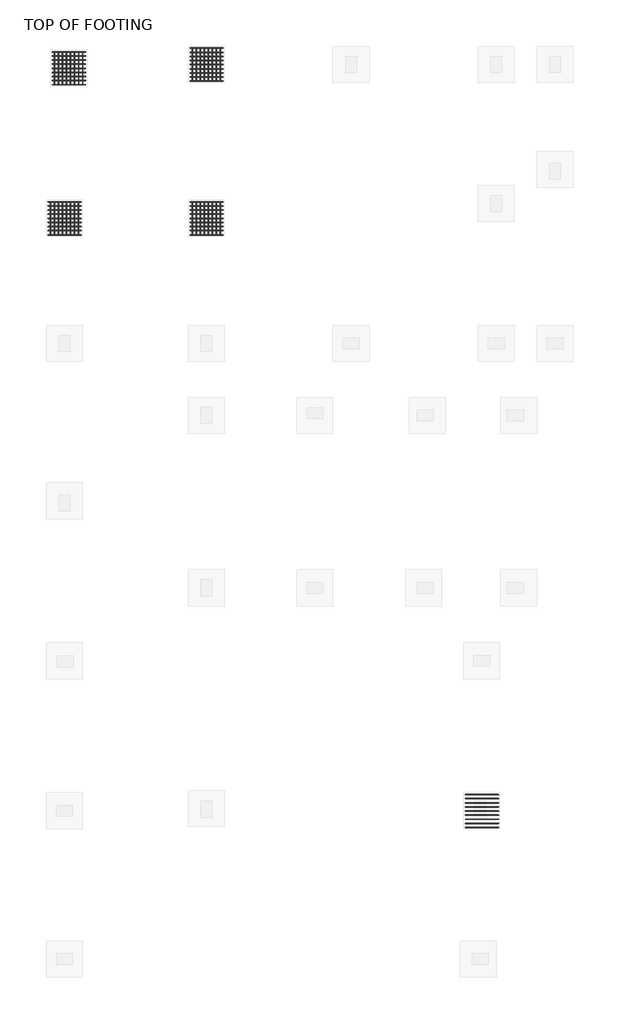
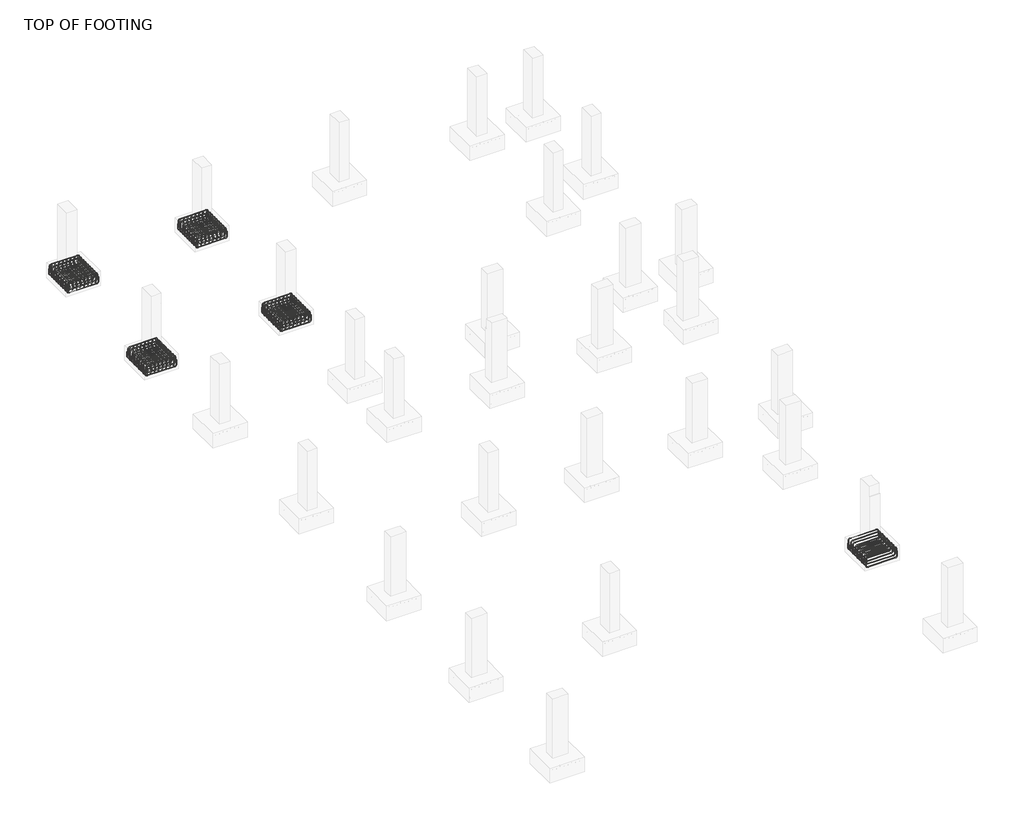
# One storey, part 13 of 20: 18 reinforcing bars.
"""IFC4 building model written with IfcOpenShell, lengths in millimetres."""

from ifc_helpers import new_model, si_unit, point, frame, origin, place, context, project, spatial, polyline, circle_curve, trimmed, segment, composite_curve, source, transform, mapped, element, save
from ifc_brep_helpers import swept_disk

model = new_model("IFC4")

# Units and contexts
model_context = context("Model", 3, world=origin())
ifc_project = project(units=[si_unit("LENGTHUNIT", "METRE", prefix="MILLI")], contexts=[model_context])

# Site, building, storey
site = spatial("IfcSite", under=ifc_project)
building = spatial("IfcBuilding", under=site)
storey = spatial("IfcBuildingStorey", under=building, Name="TOP OF FOOTING", Elevation=-1828.8)

# Reinforcing bars
placement = place(None, origin())
reinforcing_bar_shape = source(origin(), model_context, "Body", "SolidModel", [
    swept_disk(composite_curve([segment(polyline([(-5168.1365686, 22041.4849362, -2006.6587682), (-5168.1365686, 22041.4849362, -2153.9587682)]), True, "CONTINUOUS"), segment(trimmed(circle_curve(frame((-5214.4865686, 22041.4849362, -2153.9587682), z_axis=(0.0, 1.0, 0.0), x_axis=(46.350000000000364, 0.0, 0.0)), 46.35), [point((-5168.1365686, 22041.4849362, -2153.9587682))], [point((-5214.4865686, 22041.4849362, -2200.3087682))], True, "CARTESIAN"), True, "CONTINUOUS"), segment(polyline([(-5214.4865686, 22041.4849362, -2200.3087682), (-6029.0865686, 22041.4849362, -2200.3087682)]), True, "CONTINUOUS"), segment(trimmed(circle_curve(frame((-6029.0865686, 22041.4849362, -2153.9587682), z_axis=(0.0, 1.0, 0.0), x_axis=(0.0, 0.0, -46.34999999999991)), 46.35), [point((-6029.0865686, 22041.4849362, -2200.3087682))], [point((-6075.4365686, 22041.4849362, -2153.9587682))], True, "CARTESIAN"), True, "CONTINUOUS"), segment(polyline([(-6075.4365686, 22041.4849362, -2153.9587682), (-6075.4365686, 22041.4849362, -2006.6587682)]), True, "CONTINUOUS")], self_intersect=False), 6.35),
])
element("IfcReinforcingBar", 1, at=placement, inside=storey, context=model_context, shape_type="MappedRepresentation", body=[
    mapped(reinforcing_bar_shape, transform((0.0, 0.0, 0.0), x_axis=(1.0, 0.0, 0.0), y_axis=(0.0, 1.0, 0.0), z_axis=(0.0, 0.0, 1.0))),
    mapped(reinforcing_bar_shape, transform((0.0, -113.4125, 0.0), x_axis=(1.0, 0.0, 0.0), y_axis=(0.0, 1.0, 0.0), z_axis=(0.0, 0.0, 1.0))),
    mapped(reinforcing_bar_shape, transform((0.0, -226.825, 0.0), x_axis=(1.0, 0.0, 0.0), y_axis=(0.0, 1.0, 0.0), z_axis=(0.0, 0.0, 1.0))),
    mapped(reinforcing_bar_shape, transform((0.0, -340.2375, 0.0), x_axis=(1.0, 0.0, 0.0), y_axis=(0.0, 1.0, 0.0), z_axis=(0.0, 0.0, 1.0))),
    mapped(reinforcing_bar_shape, transform((0.0, -453.65, 0.0), x_axis=(1.0, 0.0, 0.0), y_axis=(0.0, 1.0, 0.0), z_axis=(0.0, 0.0, 1.0))),
    mapped(reinforcing_bar_shape, transform((0.0, -567.0625, 0.0), x_axis=(1.0, 0.0, 0.0), y_axis=(0.0, 1.0, 0.0), z_axis=(0.0, 0.0, 1.0))),
    mapped(reinforcing_bar_shape, transform((0.0, -680.475, 0.0), x_axis=(1.0, 0.0, 0.0), y_axis=(0.0, 1.0, 0.0), z_axis=(0.0, 0.0, 1.0))),
    mapped(reinforcing_bar_shape, transform((0.0, -793.8875, 0.0), x_axis=(1.0, 0.0, 0.0), y_axis=(0.0, 1.0, 0.0), z_axis=(0.0, 0.0, 1.0))),
    mapped(reinforcing_bar_shape, transform((0.0, -907.3, 0.0), x_axis=(1.0, 0.0, 0.0), y_axis=(0.0, 1.0, 0.0), z_axis=(0.0, 0.0, 1.0))),
])
reinforcing_bar_2_shape = source(origin(), model_context, "Body", "SolidModel", [
    swept_disk(composite_curve([segment(polyline([(-6055.9624573, 22041.4849362, -2068.8), (-6055.9624573, 22041.4849362, -1921.5)]), True, "CONTINUOUS"), segment(trimmed(circle_curve(frame((-6009.6124573, 22041.4849362, -1921.5), z_axis=(0.0, 1.0, 0.0), x_axis=(-46.350000000000364, 0.0, 0.0)), 46.35), [point((-6055.9624573, 22041.4849362, -1921.5))], [point((-6009.6124573, 22041.4849362, -1875.15))], True, "CARTESIAN"), True, "CONTINUOUS"), segment(polyline([(-6009.6124573, 22041.4849362, -1875.15), (-5240.1490576, 22041.4849362, -1875.15)]), True, "CONTINUOUS"), segment(trimmed(circle_curve(frame((-5240.1490576, 22041.4849362, -1921.5), z_axis=(0.0, 1.0, 0.0), x_axis=(0.0, 0.0, 46.34999999999991)), 46.35), [point((-5240.1490576, 22041.4849362, -1875.15))], [point((-5193.7990576, 22041.4849362, -1921.5))], True, "CARTESIAN"), True, "CONTINUOUS"), segment(polyline([(-5193.7990576, 22041.4849362, -1921.5), (-5193.7990576, 22041.4849362, -2068.8)]), True, "CONTINUOUS")], self_intersect=False), 6.35),
])
element("IfcReinforcingBar", 2, at=placement, inside=storey, context=model_context, shape_type="MappedRepresentation", body=[
    mapped(reinforcing_bar_2_shape, transform((0.0, 0.0, 0.0), x_axis=(1.0, 0.0, 0.0), y_axis=(0.0, 1.0, 0.0), z_axis=(0.0, 0.0, 1.0))),
    mapped(reinforcing_bar_2_shape, transform((0.0, -113.4125, 0.0), x_axis=(1.0, 0.0, 0.0), y_axis=(0.0, 1.0, 0.0), z_axis=(0.0, 0.0, 1.0))),
    mapped(reinforcing_bar_2_shape, transform((0.0, -226.825, 0.0), x_axis=(1.0, 0.0, 0.0), y_axis=(0.0, 1.0, 0.0), z_axis=(0.0, 0.0, 1.0))),
    mapped(reinforcing_bar_2_shape, transform((0.0, -340.2375, 0.0), x_axis=(1.0, 0.0, 0.0), y_axis=(0.0, 1.0, 0.0), z_axis=(0.0, 0.0, 1.0))),
    mapped(reinforcing_bar_2_shape, transform((0.0, -453.65, 0.0), x_axis=(1.0, 0.0, 0.0), y_axis=(0.0, 1.0, 0.0), z_axis=(0.0, 0.0, 1.0))),
    mapped(reinforcing_bar_2_shape, transform((0.0, -567.0625, 0.0), x_axis=(1.0, 0.0, 0.0), y_axis=(0.0, 1.0, 0.0), z_axis=(0.0, 0.0, 1.0))),
    mapped(reinforcing_bar_2_shape, transform((0.0, -680.475, 0.0), x_axis=(1.0, 0.0, 0.0), y_axis=(0.0, 1.0, 0.0), z_axis=(0.0, 0.0, 1.0))),
    mapped(reinforcing_bar_2_shape, transform((0.0, -793.8875, 0.0), x_axis=(1.0, 0.0, 0.0), y_axis=(0.0, 1.0, 0.0), z_axis=(0.0, 0.0, 1.0))),
    mapped(reinforcing_bar_2_shape, transform((0.0, -907.3, 0.0), x_axis=(1.0, 0.0, 0.0), y_axis=(0.0, 1.0, 0.0), z_axis=(0.0, 0.0, 1.0))),
])
reinforcing_bar_3_shape = source(origin(), model_context, "Body", "SolidModel", [
    swept_disk(composite_curve([segment(polyline([(-5239.63353, 22041.4849362, -2086.1951968), (-5239.63353, 22041.4849362, -1938.8951968)]), True, "CONTINUOUS"), segment(trimmed(circle_curve(frame((-5239.63353, 21995.1349362, -1938.8951968), z_axis=(1.0, 0.0, 0.0), x_axis=(0.0, 46.349999999998545, 0.0)), 46.35), [point((-5239.63353, 22041.4849362, -1938.8951968))], [point((-5239.63353, 21995.1349362, -1892.5451968))], True, "CARTESIAN"), True, "CONTINUOUS"), segment(polyline([(-5239.63353, 21995.1349362, -1892.5451968), (-5239.63353, 21180.5349362, -1892.5451968)]), True, "CONTINUOUS"), segment(trimmed(circle_curve(frame((-5239.63353, 21180.5349362, -1938.8951968), z_axis=(1.0, 0.0, 0.0), x_axis=(0.0, 0.0, 46.34999999999991)), 46.35), [point((-5239.63353, 21180.5349362, -1892.5451968))], [point((-5239.63353, 21134.1849362, -1938.8951968))], True, "CARTESIAN"), True, "CONTINUOUS"), segment(polyline([(-5239.63353, 21134.1849362, -1938.8951968), (-5239.63353, 21134.1849362, -2086.1951968)]), True, "CONTINUOUS")], self_intersect=False), 6.35),
])
element("IfcReinforcingBar", 3, at=placement, inside=storey, context=model_context, shape_type="MappedRepresentation", body=[
    mapped(reinforcing_bar_3_shape, transform((0.0, 0.0, 0.0), x_axis=(1.0, 0.0, 0.0), y_axis=(0.0, 1.0, 0.0), z_axis=(0.0, 0.0, 1.0))),
    mapped(reinforcing_bar_3_shape, transform((-111.2862402, 0.0, 0.0), x_axis=(1.0, 0.0, 0.0), y_axis=(0.0, 1.0, 0.0), z_axis=(0.0, 0.0, 1.0))),
    mapped(reinforcing_bar_3_shape, transform((-222.5724804, 0.0, 0.0), x_axis=(1.0, 0.0, 0.0), y_axis=(0.0, 1.0, 0.0), z_axis=(0.0, 0.0, 1.0))),
    mapped(reinforcing_bar_3_shape, transform((-333.8587205, 0.0, 0.0), x_axis=(1.0, 0.0, 0.0), y_axis=(0.0, 1.0, 0.0), z_axis=(0.0, 0.0, 1.0))),
    mapped(reinforcing_bar_3_shape, transform((-445.1449607, 0.0, 0.0), x_axis=(1.0, 0.0, 0.0), y_axis=(0.0, 1.0, 0.0), z_axis=(0.0, 0.0, 1.0))),
    mapped(reinforcing_bar_3_shape, transform((-556.4312009, 0.0, 0.0), x_axis=(1.0, 0.0, 0.0), y_axis=(0.0, 1.0, 0.0), z_axis=(0.0, 0.0, 1.0))),
    mapped(reinforcing_bar_3_shape, transform((-667.7174411, 0.0, 0.0), x_axis=(1.0, 0.0, 0.0), y_axis=(0.0, 1.0, 0.0), z_axis=(0.0, 0.0, 1.0))),
    mapped(reinforcing_bar_3_shape, transform((-779.0036813, 0.0, 0.0), x_axis=(1.0, 0.0, 0.0), y_axis=(0.0, 1.0, 0.0), z_axis=(0.0, 0.0, 1.0))),
])
reinforcing_bar_4_shape = source(origin(), model_context, "Body", "SolidModel", [
    swept_disk(composite_curve([segment(polyline([(-6018.6372113, 22041.4849362, -1979.1645013), (-6018.6372113, 22041.4849362, -2126.4645013)]), True, "CONTINUOUS"), segment(trimmed(circle_curve(frame((-6018.6372113, 21995.1349362, -2126.4645013), z_axis=(-1.0, 0.0, 0.0), x_axis=(0.0, 46.349999999998545, 0.0)), 46.35), [point((-6018.6372113, 22041.4849362, -2126.4645013))], [point((-6018.6372113, 21995.1349362, -2172.8145013))], True, "CARTESIAN"), True, "CONTINUOUS"), segment(polyline([(-6018.6372113, 21995.1349362, -2172.8145013), (-6018.6372113, 21180.5349362, -2172.8145013)]), True, "CONTINUOUS"), segment(trimmed(circle_curve(frame((-6018.6372113, 21180.5349362, -2126.4645013), z_axis=(-1.0, 0.0, 0.0), x_axis=(0.0, 0.0, -46.34999999999991)), 46.35), [point((-6018.6372113, 21180.5349362, -2172.8145013))], [point((-6018.6372113, 21134.1849362, -2126.4645013))], True, "CARTESIAN"), True, "CONTINUOUS"), segment(polyline([(-6018.6372113, 21134.1849362, -2126.4645013), (-6018.6372113, 21134.1849362, -1979.1645013)]), True, "CONTINUOUS")], self_intersect=False), 6.35),
])
element("IfcReinforcingBar", 4, at=placement, inside=storey, context=model_context, shape_type="MappedRepresentation", body=[
    mapped(reinforcing_bar_4_shape, transform((0.0, 0.0, 0.0), x_axis=(1.0, 0.0, 0.0), y_axis=(0.0, 1.0, 0.0), z_axis=(0.0, 0.0, 1.0))),
    mapped(reinforcing_bar_4_shape, transform((111.2862402, 0.0, 0.0), x_axis=(1.0, 0.0, 0.0), y_axis=(0.0, 1.0, 0.0), z_axis=(0.0, 0.0, 1.0))),
    mapped(reinforcing_bar_4_shape, transform((222.5724804, 0.0, 0.0), x_axis=(1.0, 0.0, 0.0), y_axis=(0.0, 1.0, 0.0), z_axis=(0.0, 0.0, 1.0))),
    mapped(reinforcing_bar_4_shape, transform((333.8587205, 0.0, 0.0), x_axis=(1.0, 0.0, 0.0), y_axis=(0.0, 1.0, 0.0), z_axis=(0.0, 0.0, 1.0))),
    mapped(reinforcing_bar_4_shape, transform((445.1449607, 0.0, 0.0), x_axis=(1.0, 0.0, 0.0), y_axis=(0.0, 1.0, 0.0), z_axis=(0.0, 0.0, 1.0))),
    mapped(reinforcing_bar_4_shape, transform((556.4312009, 0.0, 0.0), x_axis=(1.0, 0.0, 0.0), y_axis=(0.0, 1.0, 0.0), z_axis=(0.0, 0.0, 1.0))),
    mapped(reinforcing_bar_4_shape, transform((667.7174411, 0.0, 0.0), x_axis=(1.0, 0.0, 0.0), y_axis=(0.0, 1.0, 0.0), z_axis=(0.0, 0.0, 1.0))),
    mapped(reinforcing_bar_4_shape, transform((779.0036813, 0.0, 0.0), x_axis=(1.0, 0.0, 0.0), y_axis=(0.0, 1.0, 0.0), z_axis=(0.0, 0.0, 1.0))),
])
reinforcing_bar_5_shape = source(origin(), model_context, "Body", "SolidModel", [
    swept_disk(composite_curve([segment(polyline([(-1368.1365686, 22141.4849362, -2006.6587682), (-1368.1365686, 22141.4849362, -2153.9587682)]), True, "CONTINUOUS"), segment(trimmed(circle_curve(frame((-1414.4865686, 22141.4849362, -2153.9587682), z_axis=(0.0, 1.0, 0.0), x_axis=(46.350000000000136, 0.0, 0.0)), 46.35), [point((-1368.1365686, 22141.4849362, -2153.9587682))], [point((-1414.4865686, 22141.4849362, -2200.3087682))], True, "CARTESIAN"), True, "CONTINUOUS"), segment(polyline([(-1414.4865686, 22141.4849362, -2200.3087682), (-2229.0865686, 22141.4849362, -2200.3087682)]), True, "CONTINUOUS"), segment(trimmed(circle_curve(frame((-2229.0865686, 22141.4849362, -2153.9587682), z_axis=(0.0, 1.0, 0.0), x_axis=(0.0, 0.0, -46.34999999999991)), 46.35), [point((-2229.0865686, 22141.4849362, -2200.3087682))], [point((-2275.4365686, 22141.4849362, -2153.9587682))], True, "CARTESIAN"), True, "CONTINUOUS"), segment(polyline([(-2275.4365686, 22141.4849362, -2153.9587682), (-2275.4365686, 22141.4849362, -2006.6587682)]), True, "CONTINUOUS")], self_intersect=False), 6.35),
])
element("IfcReinforcingBar", 5, at=placement, inside=storey, context=model_context, shape_type="MappedRepresentation", body=[
    mapped(reinforcing_bar_5_shape, transform((0.0, 0.0, 0.0), x_axis=(1.0, 0.0, 0.0), y_axis=(0.0, 1.0, 0.0), z_axis=(0.0, 0.0, 1.0))),
    mapped(reinforcing_bar_5_shape, transform((0.0, -113.4125, 0.0), x_axis=(1.0, 0.0, 0.0), y_axis=(0.0, 1.0, 0.0), z_axis=(0.0, 0.0, 1.0))),
    mapped(reinforcing_bar_5_shape, transform((0.0, -226.825, 0.0), x_axis=(1.0, 0.0, 0.0), y_axis=(0.0, 1.0, 0.0), z_axis=(0.0, 0.0, 1.0))),
    mapped(reinforcing_bar_5_shape, transform((0.0, -340.2375, 0.0), x_axis=(1.0, 0.0, 0.0), y_axis=(0.0, 1.0, 0.0), z_axis=(0.0, 0.0, 1.0))),
    mapped(reinforcing_bar_5_shape, transform((0.0, -453.65, 0.0), x_axis=(1.0, 0.0, 0.0), y_axis=(0.0, 1.0, 0.0), z_axis=(0.0, 0.0, 1.0))),
    mapped(reinforcing_bar_5_shape, transform((0.0, -567.0625, 0.0), x_axis=(1.0, 0.0, 0.0), y_axis=(0.0, 1.0, 0.0), z_axis=(0.0, 0.0, 1.0))),
    mapped(reinforcing_bar_5_shape, transform((0.0, -680.475, 0.0), x_axis=(1.0, 0.0, 0.0), y_axis=(0.0, 1.0, 0.0), z_axis=(0.0, 0.0, 1.0))),
    mapped(reinforcing_bar_5_shape, transform((0.0, -793.8875, 0.0), x_axis=(1.0, 0.0, 0.0), y_axis=(0.0, 1.0, 0.0), z_axis=(0.0, 0.0, 1.0))),
    mapped(reinforcing_bar_5_shape, transform((0.0, -907.3, 0.0), x_axis=(1.0, 0.0, 0.0), y_axis=(0.0, 1.0, 0.0), z_axis=(0.0, 0.0, 1.0))),
])
reinforcing_bar_6_shape = source(origin(), model_context, "Body", "SolidModel", [
    swept_disk(composite_curve([segment(polyline([(-2255.9624573, 22141.4849362, -2068.8), (-2255.9624573, 22141.4849362, -1921.5)]), True, "CONTINUOUS"), segment(trimmed(circle_curve(frame((-2209.6124573, 22141.4849362, -1921.5), z_axis=(0.0, 1.0, 0.0), x_axis=(-46.34999999999991, 0.0, 0.0)), 46.35), [point((-2255.9624573, 22141.4849362, -1921.5))], [point((-2209.6124573, 22141.4849362, -1875.15))], True, "CARTESIAN"), True, "CONTINUOUS"), segment(polyline([(-2209.6124573, 22141.4849362, -1875.15), (-1440.1490576, 22141.4849362, -1875.15)]), True, "CONTINUOUS"), segment(trimmed(circle_curve(frame((-1440.1490576, 22141.4849362, -1921.5), z_axis=(0.0, 1.0, 0.0), x_axis=(0.0, 0.0, 46.34999999999991)), 46.35), [point((-1440.1490576, 22141.4849362, -1875.15))], [point((-1393.7990576, 22141.4849362, -1921.5))], True, "CARTESIAN"), True, "CONTINUOUS"), segment(polyline([(-1393.7990576, 22141.4849362, -1921.5), (-1393.7990576, 22141.4849362, -2068.8)]), True, "CONTINUOUS")], self_intersect=False), 6.35),
])
element("IfcReinforcingBar", 6, at=placement, inside=storey, context=model_context, shape_type="MappedRepresentation", body=[
    mapped(reinforcing_bar_6_shape, transform((0.0, 0.0, 0.0), x_axis=(1.0, 0.0, 0.0), y_axis=(0.0, 1.0, 0.0), z_axis=(0.0, 0.0, 1.0))),
    mapped(reinforcing_bar_6_shape, transform((0.0, -113.4125, 0.0), x_axis=(1.0, 0.0, 0.0), y_axis=(0.0, 1.0, 0.0), z_axis=(0.0, 0.0, 1.0))),
    mapped(reinforcing_bar_6_shape, transform((0.0, -226.825, 0.0), x_axis=(1.0, 0.0, 0.0), y_axis=(0.0, 1.0, 0.0), z_axis=(0.0, 0.0, 1.0))),
    mapped(reinforcing_bar_6_shape, transform((0.0, -340.2375, 0.0), x_axis=(1.0, 0.0, 0.0), y_axis=(0.0, 1.0, 0.0), z_axis=(0.0, 0.0, 1.0))),
    mapped(reinforcing_bar_6_shape, transform((0.0, -453.65, 0.0), x_axis=(1.0, 0.0, 0.0), y_axis=(0.0, 1.0, 0.0), z_axis=(0.0, 0.0, 1.0))),
    mapped(reinforcing_bar_6_shape, transform((0.0, -567.0625, 0.0), x_axis=(1.0, 0.0, 0.0), y_axis=(0.0, 1.0, 0.0), z_axis=(0.0, 0.0, 1.0))),
    mapped(reinforcing_bar_6_shape, transform((0.0, -680.475, 0.0), x_axis=(1.0, 0.0, 0.0), y_axis=(0.0, 1.0, 0.0), z_axis=(0.0, 0.0, 1.0))),
    mapped(reinforcing_bar_6_shape, transform((0.0, -793.8875, 0.0), x_axis=(1.0, 0.0, 0.0), y_axis=(0.0, 1.0, 0.0), z_axis=(0.0, 0.0, 1.0))),
    mapped(reinforcing_bar_6_shape, transform((0.0, -907.3, 0.0), x_axis=(1.0, 0.0, 0.0), y_axis=(0.0, 1.0, 0.0), z_axis=(0.0, 0.0, 1.0))),
])
reinforcing_bar_7_shape = source(origin(), model_context, "Body", "SolidModel", [
    swept_disk(composite_curve([segment(polyline([(-1439.63353, 22141.4849362, -2086.1951968), (-1439.63353, 22141.4849362, -1938.8951968)]), True, "CONTINUOUS"), segment(trimmed(circle_curve(frame((-1439.63353, 22095.1349362, -1938.8951968), z_axis=(1.0, 0.0, 0.0), x_axis=(0.0, 46.349999999998545, 0.0)), 46.35), [point((-1439.63353, 22141.4849362, -1938.8951968))], [point((-1439.63353, 22095.1349362, -1892.5451968))], True, "CARTESIAN"), True, "CONTINUOUS"), segment(polyline([(-1439.63353, 22095.1349362, -1892.5451968), (-1439.63353, 21280.5349362, -1892.5451968)]), True, "CONTINUOUS"), segment(trimmed(circle_curve(frame((-1439.63353, 21280.5349362, -1938.8951968), z_axis=(1.0, 0.0, 0.0), x_axis=(0.0, 0.0, 46.34999999999991)), 46.35), [point((-1439.63353, 21280.5349362, -1892.5451968))], [point((-1439.63353, 21234.1849362, -1938.8951968))], True, "CARTESIAN"), True, "CONTINUOUS"), segment(polyline([(-1439.63353, 21234.1849362, -1938.8951968), (-1439.63353, 21234.1849362, -2086.1951968)]), True, "CONTINUOUS")], self_intersect=False), 6.35),
])
element("IfcReinforcingBar", 7, at=placement, inside=storey, context=model_context, shape_type="MappedRepresentation", body=[
    mapped(reinforcing_bar_7_shape, transform((0.0, 0.0, 0.0), x_axis=(1.0, 0.0, 0.0), y_axis=(0.0, 1.0, 0.0), z_axis=(0.0, 0.0, 1.0))),
    mapped(reinforcing_bar_7_shape, transform((-111.2862402, 0.0, 0.0), x_axis=(1.0, 0.0, 0.0), y_axis=(0.0, 1.0, 0.0), z_axis=(0.0, 0.0, 1.0))),
    mapped(reinforcing_bar_7_shape, transform((-222.5724804, 0.0, 0.0), x_axis=(1.0, 0.0, 0.0), y_axis=(0.0, 1.0, 0.0), z_axis=(0.0, 0.0, 1.0))),
    mapped(reinforcing_bar_7_shape, transform((-333.8587205, 0.0, 0.0), x_axis=(1.0, 0.0, 0.0), y_axis=(0.0, 1.0, 0.0), z_axis=(0.0, 0.0, 1.0))),
    mapped(reinforcing_bar_7_shape, transform((-445.1449607, 0.0, 0.0), x_axis=(1.0, 0.0, 0.0), y_axis=(0.0, 1.0, 0.0), z_axis=(0.0, 0.0, 1.0))),
    mapped(reinforcing_bar_7_shape, transform((-556.4312009, 0.0, 0.0), x_axis=(1.0, 0.0, 0.0), y_axis=(0.0, 1.0, 0.0), z_axis=(0.0, 0.0, 1.0))),
    mapped(reinforcing_bar_7_shape, transform((-667.7174411, 0.0, 0.0), x_axis=(1.0, 0.0, 0.0), y_axis=(0.0, 1.0, 0.0), z_axis=(0.0, 0.0, 1.0))),
    mapped(reinforcing_bar_7_shape, transform((-779.0036813, 0.0, 0.0), x_axis=(1.0, 0.0, 0.0), y_axis=(0.0, 1.0, 0.0), z_axis=(0.0, 0.0, 1.0))),
])
reinforcing_bar_8_shape = source(origin(), model_context, "Body", "SolidModel", [
    swept_disk(composite_curve([segment(polyline([(-2218.6372113, 22141.4849362, -1979.1645013), (-2218.6372113, 22141.4849362, -2126.4645013)]), True, "CONTINUOUS"), segment(trimmed(circle_curve(frame((-2218.6372113, 22095.1349362, -2126.4645013), z_axis=(-1.0, 0.0, 0.0), x_axis=(0.0, 46.349999999998545, 0.0)), 46.35), [point((-2218.6372113, 22141.4849362, -2126.4645013))], [point((-2218.6372113, 22095.1349362, -2172.8145013))], True, "CARTESIAN"), True, "CONTINUOUS"), segment(polyline([(-2218.6372113, 22095.1349362, -2172.8145013), (-2218.6372113, 21280.5349362, -2172.8145013)]), True, "CONTINUOUS"), segment(trimmed(circle_curve(frame((-2218.6372113, 21280.5349362, -2126.4645013), z_axis=(-1.0, 0.0, 0.0), x_axis=(0.0, 0.0, -46.34999999999991)), 46.35), [point((-2218.6372113, 21280.5349362, -2172.8145013))], [point((-2218.6372113, 21234.1849362, -2126.4645013))], True, "CARTESIAN"), True, "CONTINUOUS"), segment(polyline([(-2218.6372113, 21234.1849362, -2126.4645013), (-2218.6372113, 21234.1849362, -1979.1645013)]), True, "CONTINUOUS")], self_intersect=False), 6.35),
])
element("IfcReinforcingBar", 8, at=placement, inside=storey, context=model_context, shape_type="MappedRepresentation", body=[
    mapped(reinforcing_bar_8_shape, transform((0.0, 0.0, 0.0), x_axis=(1.0, 0.0, 0.0), y_axis=(0.0, 1.0, 0.0), z_axis=(0.0, 0.0, 1.0))),
    mapped(reinforcing_bar_8_shape, transform((111.2862402, 0.0, 0.0), x_axis=(1.0, 0.0, 0.0), y_axis=(0.0, 1.0, 0.0), z_axis=(0.0, 0.0, 1.0))),
    mapped(reinforcing_bar_8_shape, transform((222.5724804, 0.0, 0.0), x_axis=(1.0, 0.0, 0.0), y_axis=(0.0, 1.0, 0.0), z_axis=(0.0, 0.0, 1.0))),
    mapped(reinforcing_bar_8_shape, transform((333.8587205, 0.0, 0.0), x_axis=(1.0, 0.0, 0.0), y_axis=(0.0, 1.0, 0.0), z_axis=(0.0, 0.0, 1.0))),
    mapped(reinforcing_bar_8_shape, transform((445.1449607, 0.0, 0.0), x_axis=(1.0, 0.0, 0.0), y_axis=(0.0, 1.0, 0.0), z_axis=(0.0, 0.0, 1.0))),
    mapped(reinforcing_bar_8_shape, transform((556.4312009, 0.0, 0.0), x_axis=(1.0, 0.0, 0.0), y_axis=(0.0, 1.0, 0.0), z_axis=(0.0, 0.0, 1.0))),
    mapped(reinforcing_bar_8_shape, transform((667.7174411, 0.0, 0.0), x_axis=(1.0, 0.0, 0.0), y_axis=(0.0, 1.0, 0.0), z_axis=(0.0, 0.0, 1.0))),
    mapped(reinforcing_bar_8_shape, transform((779.0036813, 0.0, 0.0), x_axis=(1.0, 0.0, 0.0), y_axis=(0.0, 1.0, 0.0), z_axis=(0.0, 0.0, 1.0))),
])
reinforcing_bar_9_shape = source(origin(), model_context, "Body", "SolidModel", [
    swept_disk(composite_curve([segment(polyline([(-1368.1365686, 17903.3648651, -2006.6587682), (-1368.1365686, 17903.3648651, -2153.9587682)]), True, "CONTINUOUS"), segment(trimmed(circle_curve(frame((-1414.4865686, 17903.3648651, -2153.9587682), z_axis=(0.0, 1.0, 0.0), x_axis=(46.350000000000136, 0.0, 0.0)), 46.35), [point((-1368.1365686, 17903.3648651, -2153.9587682))], [point((-1414.4865686, 17903.3648651, -2200.3087682))], True, "CARTESIAN"), True, "CONTINUOUS"), segment(polyline([(-1414.4865686, 17903.3648651, -2200.3087682), (-2229.0865686, 17903.3648651, -2200.3087682)]), True, "CONTINUOUS"), segment(trimmed(circle_curve(frame((-2229.0865686, 17903.3648651, -2153.9587682), z_axis=(0.0, 1.0, 0.0), x_axis=(0.0, 0.0, -46.34999999999991)), 46.35), [point((-2229.0865686, 17903.3648651, -2200.3087682))], [point((-2275.4365686, 17903.3648651, -2153.9587682))], True, "CARTESIAN"), True, "CONTINUOUS"), segment(polyline([(-2275.4365686, 17903.3648651, -2153.9587682), (-2275.4365686, 17903.3648651, -2006.6587682)]), True, "CONTINUOUS")], self_intersect=False), 6.35),
])
element("IfcReinforcingBar", 9, at=placement, inside=storey, context=model_context, shape_type="MappedRepresentation", body=[
    mapped(reinforcing_bar_9_shape, transform((0.0, 0.0, 0.0), x_axis=(1.0, 0.0, 0.0), y_axis=(0.0, 1.0, 0.0), z_axis=(0.0, 0.0, 1.0))),
    mapped(reinforcing_bar_9_shape, transform((0.0, -113.4125, 0.0), x_axis=(1.0, 0.0, 0.0), y_axis=(0.0, 1.0, 0.0), z_axis=(0.0, 0.0, 1.0))),
    mapped(reinforcing_bar_9_shape, transform((0.0, -226.825, 0.0), x_axis=(1.0, 0.0, 0.0), y_axis=(0.0, 1.0, 0.0), z_axis=(0.0, 0.0, 1.0))),
    mapped(reinforcing_bar_9_shape, transform((0.0, -340.2375, 0.0), x_axis=(1.0, 0.0, 0.0), y_axis=(0.0, 1.0, 0.0), z_axis=(0.0, 0.0, 1.0))),
    mapped(reinforcing_bar_9_shape, transform((0.0, -453.65, 0.0), x_axis=(1.0, 0.0, 0.0), y_axis=(0.0, 1.0, 0.0), z_axis=(0.0, 0.0, 1.0))),
    mapped(reinforcing_bar_9_shape, transform((0.0, -567.0625, 0.0), x_axis=(1.0, 0.0, 0.0), y_axis=(0.0, 1.0, 0.0), z_axis=(0.0, 0.0, 1.0))),
    mapped(reinforcing_bar_9_shape, transform((0.0, -680.475, 0.0), x_axis=(1.0, 0.0, 0.0), y_axis=(0.0, 1.0, 0.0), z_axis=(0.0, 0.0, 1.0))),
    mapped(reinforcing_bar_9_shape, transform((0.0, -793.8875, 0.0), x_axis=(1.0, 0.0, 0.0), y_axis=(0.0, 1.0, 0.0), z_axis=(0.0, 0.0, 1.0))),
    mapped(reinforcing_bar_9_shape, transform((0.0, -907.3, 0.0), x_axis=(1.0, 0.0, 0.0), y_axis=(0.0, 1.0, 0.0), z_axis=(0.0, 0.0, 1.0))),
])
reinforcing_bar_10_shape = source(origin(), model_context, "Body", "SolidModel", [
    swept_disk(composite_curve([segment(polyline([(-2255.9624573, 17903.3648651, -2068.8), (-2255.9624573, 17903.3648651, -1921.5)]), True, "CONTINUOUS"), segment(trimmed(circle_curve(frame((-2209.6124573, 17903.3648651, -1921.5), z_axis=(0.0, 1.0, 0.0), x_axis=(-46.34999999999991, 0.0, 0.0)), 46.35), [point((-2255.9624573, 17903.3648651, -1921.5))], [point((-2209.6124573, 17903.3648651, -1875.15))], True, "CARTESIAN"), True, "CONTINUOUS"), segment(polyline([(-2209.6124573, 17903.3648651, -1875.15), (-1440.1490576, 17903.3648651, -1875.15)]), True, "CONTINUOUS"), segment(trimmed(circle_curve(frame((-1440.1490576, 17903.3648651, -1921.5), z_axis=(0.0, 1.0, 0.0), x_axis=(0.0, 0.0, 46.34999999999991)), 46.35), [point((-1440.1490576, 17903.3648651, -1875.15))], [point((-1393.7990576, 17903.3648651, -1921.5))], True, "CARTESIAN"), True, "CONTINUOUS"), segment(polyline([(-1393.7990576, 17903.3648651, -1921.5), (-1393.7990576, 17903.3648651, -2068.8)]), True, "CONTINUOUS")], self_intersect=False), 6.35),
])
element("IfcReinforcingBar", 10, at=placement, inside=storey, context=model_context, shape_type="MappedRepresentation", body=[
    mapped(reinforcing_bar_10_shape, transform((0.0, 0.0, 0.0), x_axis=(1.0, 0.0, 0.0), y_axis=(0.0, 1.0, 0.0), z_axis=(0.0, 0.0, 1.0))),
    mapped(reinforcing_bar_10_shape, transform((0.0, -113.4125, 0.0), x_axis=(1.0, 0.0, 0.0), y_axis=(0.0, 1.0, 0.0), z_axis=(0.0, 0.0, 1.0))),
    mapped(reinforcing_bar_10_shape, transform((0.0, -226.825, 0.0), x_axis=(1.0, 0.0, 0.0), y_axis=(0.0, 1.0, 0.0), z_axis=(0.0, 0.0, 1.0))),
    mapped(reinforcing_bar_10_shape, transform((0.0, -340.2375, 0.0), x_axis=(1.0, 0.0, 0.0), y_axis=(0.0, 1.0, 0.0), z_axis=(0.0, 0.0, 1.0))),
    mapped(reinforcing_bar_10_shape, transform((0.0, -453.65, 0.0), x_axis=(1.0, 0.0, 0.0), y_axis=(0.0, 1.0, 0.0), z_axis=(0.0, 0.0, 1.0))),
    mapped(reinforcing_bar_10_shape, transform((0.0, -567.0625, 0.0), x_axis=(1.0, 0.0, 0.0), y_axis=(0.0, 1.0, 0.0), z_axis=(0.0, 0.0, 1.0))),
    mapped(reinforcing_bar_10_shape, transform((0.0, -680.475, 0.0), x_axis=(1.0, 0.0, 0.0), y_axis=(0.0, 1.0, 0.0), z_axis=(0.0, 0.0, 1.0))),
    mapped(reinforcing_bar_10_shape, transform((0.0, -793.8875, 0.0), x_axis=(1.0, 0.0, 0.0), y_axis=(0.0, 1.0, 0.0), z_axis=(0.0, 0.0, 1.0))),
    mapped(reinforcing_bar_10_shape, transform((0.0, -907.3, 0.0), x_axis=(1.0, 0.0, 0.0), y_axis=(0.0, 1.0, 0.0), z_axis=(0.0, 0.0, 1.0))),
])
reinforcing_bar_11_shape = source(origin(), model_context, "Body", "SolidModel", [
    swept_disk(composite_curve([segment(polyline([(-1439.63353, 17903.3648651, -2086.1951968), (-1439.63353, 17903.3648651, -1938.8951968)]), True, "CONTINUOUS"), segment(trimmed(circle_curve(frame((-1439.63353, 17857.0148651, -1938.8951968), z_axis=(1.0, 0.0, 0.0), x_axis=(0.0, 46.349999999998545, 0.0)), 46.35), [point((-1439.63353, 17903.3648651, -1938.8951968))], [point((-1439.63353, 17857.0148651, -1892.5451968))], True, "CARTESIAN"), True, "CONTINUOUS"), segment(polyline([(-1439.63353, 17857.0148651, -1892.5451968), (-1439.63353, 17042.4148651, -1892.5451968)]), True, "CONTINUOUS"), segment(trimmed(circle_curve(frame((-1439.63353, 17042.4148651, -1938.8951968), z_axis=(1.0, 0.0, 0.0), x_axis=(0.0, 0.0, 46.34999999999991)), 46.35), [point((-1439.63353, 17042.4148651, -1892.5451968))], [point((-1439.63353, 16996.0648651, -1938.8951968))], True, "CARTESIAN"), True, "CONTINUOUS"), segment(polyline([(-1439.63353, 16996.0648651, -1938.8951968), (-1439.63353, 16996.0648651, -2086.1951968)]), True, "CONTINUOUS")], self_intersect=False), 6.35),
])
element("IfcReinforcingBar", 11, at=placement, inside=storey, context=model_context, shape_type="MappedRepresentation", body=[
    mapped(reinforcing_bar_11_shape, transform((0.0, 0.0, 0.0), x_axis=(1.0, 0.0, 0.0), y_axis=(0.0, 1.0, 0.0), z_axis=(0.0, 0.0, 1.0))),
    mapped(reinforcing_bar_11_shape, transform((-111.2862402, 0.0, 0.0), x_axis=(1.0, 0.0, 0.0), y_axis=(0.0, 1.0, 0.0), z_axis=(0.0, 0.0, 1.0))),
    mapped(reinforcing_bar_11_shape, transform((-222.5724804, 0.0, 0.0), x_axis=(1.0, 0.0, 0.0), y_axis=(0.0, 1.0, 0.0), z_axis=(0.0, 0.0, 1.0))),
    mapped(reinforcing_bar_11_shape, transform((-333.8587205, 0.0, 0.0), x_axis=(1.0, 0.0, 0.0), y_axis=(0.0, 1.0, 0.0), z_axis=(0.0, 0.0, 1.0))),
    mapped(reinforcing_bar_11_shape, transform((-445.1449607, 0.0, 0.0), x_axis=(1.0, 0.0, 0.0), y_axis=(0.0, 1.0, 0.0), z_axis=(0.0, 0.0, 1.0))),
    mapped(reinforcing_bar_11_shape, transform((-556.4312009, 0.0, 0.0), x_axis=(1.0, 0.0, 0.0), y_axis=(0.0, 1.0, 0.0), z_axis=(0.0, 0.0, 1.0))),
    mapped(reinforcing_bar_11_shape, transform((-667.7174411, 0.0, 0.0), x_axis=(1.0, 0.0, 0.0), y_axis=(0.0, 1.0, 0.0), z_axis=(0.0, 0.0, 1.0))),
    mapped(reinforcing_bar_11_shape, transform((-779.0036813, 0.0, 0.0), x_axis=(1.0, 0.0, 0.0), y_axis=(0.0, 1.0, 0.0), z_axis=(0.0, 0.0, 1.0))),
])
reinforcing_bar_12_shape = source(origin(), model_context, "Body", "SolidModel", [
    swept_disk(composite_curve([segment(polyline([(-2218.6372113, 17903.3648651, -1979.1645013), (-2218.6372113, 17903.3648651, -2126.4645013)]), True, "CONTINUOUS"), segment(trimmed(circle_curve(frame((-2218.6372113, 17857.0148651, -2126.4645013), z_axis=(-1.0, 0.0, 0.0), x_axis=(0.0, 46.349999999998545, 0.0)), 46.35), [point((-2218.6372113, 17903.3648651, -2126.4645013))], [point((-2218.6372113, 17857.0148651, -2172.8145013))], True, "CARTESIAN"), True, "CONTINUOUS"), segment(polyline([(-2218.6372113, 17857.0148651, -2172.8145013), (-2218.6372113, 17042.4148651, -2172.8145013)]), True, "CONTINUOUS"), segment(trimmed(circle_curve(frame((-2218.6372113, 17042.4148651, -2126.4645013), z_axis=(-1.0, 0.0, 0.0), x_axis=(0.0, 0.0, -46.34999999999991)), 46.35), [point((-2218.6372113, 17042.4148651, -2172.8145013))], [point((-2218.6372113, 16996.0648651, -2126.4645013))], True, "CARTESIAN"), True, "CONTINUOUS"), segment(polyline([(-2218.6372113, 16996.0648651, -2126.4645013), (-2218.6372113, 16996.0648651, -1979.1645013)]), True, "CONTINUOUS")], self_intersect=False), 6.35),
])
element("IfcReinforcingBar", 12, at=placement, inside=storey, context=model_context, shape_type="MappedRepresentation", body=[
    mapped(reinforcing_bar_12_shape, transform((0.0, 0.0, 0.0), x_axis=(1.0, 0.0, 0.0), y_axis=(0.0, 1.0, 0.0), z_axis=(0.0, 0.0, 1.0))),
    mapped(reinforcing_bar_12_shape, transform((111.2862402, 0.0, 0.0), x_axis=(1.0, 0.0, 0.0), y_axis=(0.0, 1.0, 0.0), z_axis=(0.0, 0.0, 1.0))),
    mapped(reinforcing_bar_12_shape, transform((222.5724804, 0.0, 0.0), x_axis=(1.0, 0.0, 0.0), y_axis=(0.0, 1.0, 0.0), z_axis=(0.0, 0.0, 1.0))),
    mapped(reinforcing_bar_12_shape, transform((333.8587205, 0.0, 0.0), x_axis=(1.0, 0.0, 0.0), y_axis=(0.0, 1.0, 0.0), z_axis=(0.0, 0.0, 1.0))),
    mapped(reinforcing_bar_12_shape, transform((445.1449607, 0.0, 0.0), x_axis=(1.0, 0.0, 0.0), y_axis=(0.0, 1.0, 0.0), z_axis=(0.0, 0.0, 1.0))),
    mapped(reinforcing_bar_12_shape, transform((556.4312009, 0.0, 0.0), x_axis=(1.0, 0.0, 0.0), y_axis=(0.0, 1.0, 0.0), z_axis=(0.0, 0.0, 1.0))),
    mapped(reinforcing_bar_12_shape, transform((667.7174411, 0.0, 0.0), x_axis=(1.0, 0.0, 0.0), y_axis=(0.0, 1.0, 0.0), z_axis=(0.0, 0.0, 1.0))),
    mapped(reinforcing_bar_12_shape, transform((779.0036813, 0.0, 0.0), x_axis=(1.0, 0.0, 0.0), y_axis=(0.0, 1.0, 0.0), z_axis=(0.0, 0.0, 1.0))),
])
reinforcing_bar_13_shape = source(origin(), model_context, "Body", "SolidModel", [
    swept_disk(composite_curve([segment(polyline([(-5285.1605653, 17903.3648651, -2006.6587682), (-5285.1605653, 17903.3648651, -2153.9587682)]), True, "CONTINUOUS"), segment(trimmed(circle_curve(frame((-5331.5105653, 17903.3648651, -2153.9587682), z_axis=(0.0, 1.0, 0.0), x_axis=(46.350000000000364, 0.0, 0.0)), 46.35), [point((-5285.1605653, 17903.3648651, -2153.9587682))], [point((-5331.5105653, 17903.3648651, -2200.3087682))], True, "CARTESIAN"), True, "CONTINUOUS"), segment(polyline([(-5331.5105653, 17903.3648651, -2200.3087682), (-6146.1105653, 17903.3648651, -2200.3087682)]), True, "CONTINUOUS"), segment(trimmed(circle_curve(frame((-6146.1105653, 17903.3648651, -2153.9587682), z_axis=(0.0, 1.0, 0.0), x_axis=(0.0, 0.0, -46.34999999999991)), 46.35), [point((-6146.1105653, 17903.3648651, -2200.3087682))], [point((-6192.4605653, 17903.3648651, -2153.9587682))], True, "CARTESIAN"), True, "CONTINUOUS"), segment(polyline([(-6192.4605653, 17903.3648651, -2153.9587682), (-6192.4605653, 17903.3648651, -2006.6587682)]), True, "CONTINUOUS")], self_intersect=False), 6.35),
])
element("IfcReinforcingBar", 13, at=placement, inside=storey, context=model_context, shape_type="MappedRepresentation", body=[
    mapped(reinforcing_bar_13_shape, transform((0.0, 0.0, 0.0), x_axis=(1.0, 0.0, 0.0), y_axis=(0.0, 1.0, 0.0), z_axis=(0.0, 0.0, 1.0))),
    mapped(reinforcing_bar_13_shape, transform((0.0, -113.4125, 0.0), x_axis=(1.0, 0.0, 0.0), y_axis=(0.0, 1.0, 0.0), z_axis=(0.0, 0.0, 1.0))),
    mapped(reinforcing_bar_13_shape, transform((0.0, -226.825, 0.0), x_axis=(1.0, 0.0, 0.0), y_axis=(0.0, 1.0, 0.0), z_axis=(0.0, 0.0, 1.0))),
    mapped(reinforcing_bar_13_shape, transform((0.0, -340.2375, 0.0), x_axis=(1.0, 0.0, 0.0), y_axis=(0.0, 1.0, 0.0), z_axis=(0.0, 0.0, 1.0))),
    mapped(reinforcing_bar_13_shape, transform((0.0, -453.65, 0.0), x_axis=(1.0, 0.0, 0.0), y_axis=(0.0, 1.0, 0.0), z_axis=(0.0, 0.0, 1.0))),
    mapped(reinforcing_bar_13_shape, transform((0.0, -567.0625, 0.0), x_axis=(1.0, 0.0, 0.0), y_axis=(0.0, 1.0, 0.0), z_axis=(0.0, 0.0, 1.0))),
    mapped(reinforcing_bar_13_shape, transform((0.0, -680.475, 0.0), x_axis=(1.0, 0.0, 0.0), y_axis=(0.0, 1.0, 0.0), z_axis=(0.0, 0.0, 1.0))),
    mapped(reinforcing_bar_13_shape, transform((0.0, -793.8875, 0.0), x_axis=(1.0, 0.0, 0.0), y_axis=(0.0, 1.0, 0.0), z_axis=(0.0, 0.0, 1.0))),
    mapped(reinforcing_bar_13_shape, transform((0.0, -907.3, 0.0), x_axis=(1.0, 0.0, 0.0), y_axis=(0.0, 1.0, 0.0), z_axis=(0.0, 0.0, 1.0))),
])
reinforcing_bar_14_shape = source(origin(), model_context, "Body", "SolidModel", [
    swept_disk(composite_curve([segment(polyline([(-6172.986454, 17903.3648651, -2068.8), (-6172.986454, 17903.3648651, -1921.5)]), True, "CONTINUOUS"), segment(trimmed(circle_curve(frame((-6126.636454, 17903.3648651, -1921.5), z_axis=(0.0, 1.0, 0.0), x_axis=(-46.349999999999454, 0.0, 0.0)), 46.35), [point((-6172.986454, 17903.3648651, -1921.5))], [point((-6126.636454, 17903.3648651, -1875.15))], True, "CARTESIAN"), True, "CONTINUOUS"), segment(polyline([(-6126.636454, 17903.3648651, -1875.15), (-5357.1730543, 17903.3648651, -1875.15)]), True, "CONTINUOUS"), segment(trimmed(circle_curve(frame((-5357.1730543, 17903.3648651, -1921.5), z_axis=(0.0, 1.0, 0.0), x_axis=(0.0, 0.0, 46.34999999999991)), 46.35), [point((-5357.1730543, 17903.3648651, -1875.15))], [point((-5310.8230543, 17903.3648651, -1921.5))], True, "CARTESIAN"), True, "CONTINUOUS"), segment(polyline([(-5310.8230543, 17903.3648651, -1921.5), (-5310.8230543, 17903.3648651, -2068.8)]), True, "CONTINUOUS")], self_intersect=False), 6.35),
])
element("IfcReinforcingBar", 14, at=placement, inside=storey, context=model_context, shape_type="MappedRepresentation", body=[
    mapped(reinforcing_bar_14_shape, transform((0.0, 0.0, 0.0), x_axis=(1.0, 0.0, 0.0), y_axis=(0.0, 1.0, 0.0), z_axis=(0.0, 0.0, 1.0))),
    mapped(reinforcing_bar_14_shape, transform((0.0, -113.4125, 0.0), x_axis=(1.0, 0.0, 0.0), y_axis=(0.0, 1.0, 0.0), z_axis=(0.0, 0.0, 1.0))),
    mapped(reinforcing_bar_14_shape, transform((0.0, -226.825, 0.0), x_axis=(1.0, 0.0, 0.0), y_axis=(0.0, 1.0, 0.0), z_axis=(0.0, 0.0, 1.0))),
    mapped(reinforcing_bar_14_shape, transform((0.0, -340.2375, 0.0), x_axis=(1.0, 0.0, 0.0), y_axis=(0.0, 1.0, 0.0), z_axis=(0.0, 0.0, 1.0))),
    mapped(reinforcing_bar_14_shape, transform((0.0, -453.65, 0.0), x_axis=(1.0, 0.0, 0.0), y_axis=(0.0, 1.0, 0.0), z_axis=(0.0, 0.0, 1.0))),
    mapped(reinforcing_bar_14_shape, transform((0.0, -567.0625, 0.0), x_axis=(1.0, 0.0, 0.0), y_axis=(0.0, 1.0, 0.0), z_axis=(0.0, 0.0, 1.0))),
    mapped(reinforcing_bar_14_shape, transform((0.0, -680.475, 0.0), x_axis=(1.0, 0.0, 0.0), y_axis=(0.0, 1.0, 0.0), z_axis=(0.0, 0.0, 1.0))),
    mapped(reinforcing_bar_14_shape, transform((0.0, -793.8875, 0.0), x_axis=(1.0, 0.0, 0.0), y_axis=(0.0, 1.0, 0.0), z_axis=(0.0, 0.0, 1.0))),
    mapped(reinforcing_bar_14_shape, transform((0.0, -907.3, 0.0), x_axis=(1.0, 0.0, 0.0), y_axis=(0.0, 1.0, 0.0), z_axis=(0.0, 0.0, 1.0))),
])
reinforcing_bar_15_shape = source(origin(), model_context, "Body", "SolidModel", [
    swept_disk(composite_curve([segment(polyline([(-5356.6575267, 17903.3648651, -2086.1951968), (-5356.6575267, 17903.3648651, -1938.8951968)]), True, "CONTINUOUS"), segment(trimmed(circle_curve(frame((-5356.6575267, 17857.0148651, -1938.8951968), z_axis=(1.0, 0.0, 0.0), x_axis=(0.0, 46.349999999998545, 0.0)), 46.35), [point((-5356.6575267, 17903.3648651, -1938.8951968))], [point((-5356.6575267, 17857.0148651, -1892.5451968))], True, "CARTESIAN"), True, "CONTINUOUS"), segment(polyline([(-5356.6575267, 17857.0148651, -1892.5451968), (-5356.6575267, 17042.4148651, -1892.5451968)]), True, "CONTINUOUS"), segment(trimmed(circle_curve(frame((-5356.6575267, 17042.4148651, -1938.8951968), z_axis=(1.0, 0.0, 0.0), x_axis=(0.0, 0.0, 46.34999999999991)), 46.35), [point((-5356.6575267, 17042.4148651, -1892.5451968))], [point((-5356.6575267, 16996.0648651, -1938.8951968))], True, "CARTESIAN"), True, "CONTINUOUS"), segment(polyline([(-5356.6575267, 16996.0648651, -1938.8951968), (-5356.6575267, 16996.0648651, -2086.1951968)]), True, "CONTINUOUS")], self_intersect=False), 6.35),
])
element("IfcReinforcingBar", 15, at=placement, inside=storey, context=model_context, shape_type="MappedRepresentation", body=[
    mapped(reinforcing_bar_15_shape, transform((0.0, 0.0, 0.0), x_axis=(1.0, 0.0, 0.0), y_axis=(0.0, 1.0, 0.0), z_axis=(0.0, 0.0, 1.0))),
    mapped(reinforcing_bar_15_shape, transform((-111.2862402, 0.0, 0.0), x_axis=(1.0, 0.0, 0.0), y_axis=(0.0, 1.0, 0.0), z_axis=(0.0, 0.0, 1.0))),
    mapped(reinforcing_bar_15_shape, transform((-222.5724804, 0.0, 0.0), x_axis=(1.0, 0.0, 0.0), y_axis=(0.0, 1.0, 0.0), z_axis=(0.0, 0.0, 1.0))),
    mapped(reinforcing_bar_15_shape, transform((-333.8587205, 0.0, 0.0), x_axis=(1.0, 0.0, 0.0), y_axis=(0.0, 1.0, 0.0), z_axis=(0.0, 0.0, 1.0))),
    mapped(reinforcing_bar_15_shape, transform((-445.1449607, 0.0, 0.0), x_axis=(1.0, 0.0, 0.0), y_axis=(0.0, 1.0, 0.0), z_axis=(0.0, 0.0, 1.0))),
    mapped(reinforcing_bar_15_shape, transform((-556.4312009, 0.0, 0.0), x_axis=(1.0, 0.0, 0.0), y_axis=(0.0, 1.0, 0.0), z_axis=(0.0, 0.0, 1.0))),
    mapped(reinforcing_bar_15_shape, transform((-667.7174411, 0.0, 0.0), x_axis=(1.0, 0.0, 0.0), y_axis=(0.0, 1.0, 0.0), z_axis=(0.0, 0.0, 1.0))),
    mapped(reinforcing_bar_15_shape, transform((-779.0036813, 0.0, 0.0), x_axis=(1.0, 0.0, 0.0), y_axis=(0.0, 1.0, 0.0), z_axis=(0.0, 0.0, 1.0))),
])
reinforcing_bar_16_shape = source(origin(), model_context, "Body", "SolidModel", [
    swept_disk(composite_curve([segment(polyline([(-6135.661208, 17903.3648651, -1979.1645013), (-6135.661208, 17903.3648651, -2126.4645013)]), True, "CONTINUOUS"), segment(trimmed(circle_curve(frame((-6135.661208, 17857.0148651, -2126.4645013), z_axis=(-1.0, 0.0, 0.0), x_axis=(0.0, 46.349999999998545, 0.0)), 46.35), [point((-6135.661208, 17903.3648651, -2126.4645013))], [point((-6135.661208, 17857.0148651, -2172.8145013))], True, "CARTESIAN"), True, "CONTINUOUS"), segment(polyline([(-6135.661208, 17857.0148651, -2172.8145013), (-6135.661208, 17042.4148651, -2172.8145013)]), True, "CONTINUOUS"), segment(trimmed(circle_curve(frame((-6135.661208, 17042.4148651, -2126.4645013), z_axis=(-1.0, 0.0, 0.0), x_axis=(0.0, 0.0, -46.34999999999991)), 46.35), [point((-6135.661208, 17042.4148651, -2172.8145013))], [point((-6135.661208, 16996.0648651, -2126.4645013))], True, "CARTESIAN"), True, "CONTINUOUS"), segment(polyline([(-6135.661208, 16996.0648651, -2126.4645013), (-6135.661208, 16996.0648651, -1979.1645013)]), True, "CONTINUOUS")], self_intersect=False), 6.35),
])
element("IfcReinforcingBar", 16, at=placement, inside=storey, context=model_context, shape_type="MappedRepresentation", body=[
    mapped(reinforcing_bar_16_shape, transform((0.0, 0.0, 0.0), x_axis=(1.0, 0.0, 0.0), y_axis=(0.0, 1.0, 0.0), z_axis=(0.0, 0.0, 1.0))),
    mapped(reinforcing_bar_16_shape, transform((111.2862402, 0.0, 0.0), x_axis=(1.0, 0.0, 0.0), y_axis=(0.0, 1.0, 0.0), z_axis=(0.0, 0.0, 1.0))),
    mapped(reinforcing_bar_16_shape, transform((222.5724804, 0.0, 0.0), x_axis=(1.0, 0.0, 0.0), y_axis=(0.0, 1.0, 0.0), z_axis=(0.0, 0.0, 1.0))),
    mapped(reinforcing_bar_16_shape, transform((333.8587205, 0.0, 0.0), x_axis=(1.0, 0.0, 0.0), y_axis=(0.0, 1.0, 0.0), z_axis=(0.0, 0.0, 1.0))),
    mapped(reinforcing_bar_16_shape, transform((445.1449607, 0.0, 0.0), x_axis=(1.0, 0.0, 0.0), y_axis=(0.0, 1.0, 0.0), z_axis=(0.0, 0.0, 1.0))),
    mapped(reinforcing_bar_16_shape, transform((556.4312009, 0.0, 0.0), x_axis=(1.0, 0.0, 0.0), y_axis=(0.0, 1.0, 0.0), z_axis=(0.0, 0.0, 1.0))),
    mapped(reinforcing_bar_16_shape, transform((667.7174411, 0.0, 0.0), x_axis=(1.0, 0.0, 0.0), y_axis=(0.0, 1.0, 0.0), z_axis=(0.0, 0.0, 1.0))),
    mapped(reinforcing_bar_16_shape, transform((779.0036813, 0.0, 0.0), x_axis=(1.0, 0.0, 0.0), y_axis=(0.0, 1.0, 0.0), z_axis=(0.0, 0.0, 1.0))),
])
reinforcing_bar_17_shape = source(origin(), model_context, "Body", "SolidModel", [
    swept_disk(composite_curve([segment(polyline([(6236.1748054, 1554.8213929, -2006.6587682), (6236.1748054, 1554.8213929, -2153.9587682)]), True, "CONTINUOUS"), segment(trimmed(circle_curve(frame((6189.8248054, 1554.8213929, -2153.9587682), z_axis=(0.0, 1.0, 0.0), x_axis=(46.350000000000364, 0.0, 0.0)), 46.35), [point((6236.1748054, 1554.8213929, -2153.9587682))], [point((6189.8248054, 1554.8213929, -2200.3087682))], True, "CARTESIAN"), True, "CONTINUOUS"), segment(polyline([(6189.8248054, 1554.8213929, -2200.3087682), (5375.2248054, 1554.8213929, -2200.3087682)]), True, "CONTINUOUS"), segment(trimmed(circle_curve(frame((5375.2248054, 1554.8213929, -2153.9587682), z_axis=(0.0, 1.0, 0.0), x_axis=(0.0, 0.0, -46.34999999999991)), 46.35), [point((5375.2248054, 1554.8213929, -2200.3087682))], [point((5328.8748054, 1554.8213929, -2153.9587682))], True, "CARTESIAN"), True, "CONTINUOUS"), segment(polyline([(5328.8748054, 1554.8213929, -2153.9587682), (5328.8748054, 1554.8213929, -2006.6587682)]), True, "CONTINUOUS")], self_intersect=False), 6.35),
])
element("IfcReinforcingBar", 17, at=placement, inside=storey, context=model_context, shape_type="MappedRepresentation", body=[
    mapped(reinforcing_bar_17_shape, transform((0.0, 0.0, 0.0), x_axis=(1.0, 0.0, 0.0), y_axis=(0.0, 1.0, 0.0), z_axis=(0.0, 0.0, 1.0))),
    mapped(reinforcing_bar_17_shape, transform((0.0, -113.4125, 0.0), x_axis=(1.0, 0.0, 0.0), y_axis=(0.0, 1.0, 0.0), z_axis=(0.0, 0.0, 1.0))),
    mapped(reinforcing_bar_17_shape, transform((0.0, -226.825, 0.0), x_axis=(1.0, 0.0, 0.0), y_axis=(0.0, 1.0, 0.0), z_axis=(0.0, 0.0, 1.0))),
    mapped(reinforcing_bar_17_shape, transform((0.0, -340.2375, 0.0), x_axis=(1.0, 0.0, 0.0), y_axis=(0.0, 1.0, 0.0), z_axis=(0.0, 0.0, 1.0))),
    mapped(reinforcing_bar_17_shape, transform((0.0, -453.65, 0.0), x_axis=(1.0, 0.0, 0.0), y_axis=(0.0, 1.0, 0.0), z_axis=(0.0, 0.0, 1.0))),
    mapped(reinforcing_bar_17_shape, transform((0.0, -567.0625, 0.0), x_axis=(1.0, 0.0, 0.0), y_axis=(0.0, 1.0, 0.0), z_axis=(0.0, 0.0, 1.0))),
    mapped(reinforcing_bar_17_shape, transform((0.0, -680.475, 0.0), x_axis=(1.0, 0.0, 0.0), y_axis=(0.0, 1.0, 0.0), z_axis=(0.0, 0.0, 1.0))),
    mapped(reinforcing_bar_17_shape, transform((0.0, -793.8875, 0.0), x_axis=(1.0, 0.0, 0.0), y_axis=(0.0, 1.0, 0.0), z_axis=(0.0, 0.0, 1.0))),
    mapped(reinforcing_bar_17_shape, transform((0.0, -907.3, 0.0), x_axis=(1.0, 0.0, 0.0), y_axis=(0.0, 1.0, 0.0), z_axis=(0.0, 0.0, 1.0))),
])
reinforcing_bar_18_shape = source(origin(), model_context, "Body", "SolidModel", [
    swept_disk(composite_curve([segment(polyline([(5348.3489167, 1554.8213929, -2068.8), (5348.3489167, 1554.8213929, -1921.5)]), True, "CONTINUOUS"), segment(trimmed(circle_curve(frame((5394.6989167, 1554.8213929, -1921.5), z_axis=(0.0, 1.0, 0.0), x_axis=(-46.350000000000364, 0.0, 0.0)), 46.35), [point((5348.3489167, 1554.8213929, -1921.5))], [point((5394.6989167, 1554.8213929, -1875.15))], True, "CARTESIAN"), True, "CONTINUOUS"), segment(polyline([(5394.6989167, 1554.8213929, -1875.15), (6164.1623164, 1554.8213929, -1875.15)]), True, "CONTINUOUS"), segment(trimmed(circle_curve(frame((6164.1623164, 1554.8213929, -1921.5), z_axis=(0.0, 1.0, 0.0), x_axis=(0.0, 0.0, 46.34999999999991)), 46.35), [point((6164.1623164, 1554.8213929, -1875.15))], [point((6210.5123164, 1554.8213929, -1921.5))], True, "CARTESIAN"), True, "CONTINUOUS"), segment(polyline([(6210.5123164, 1554.8213929, -1921.5), (6210.5123164, 1554.8213929, -2068.8)]), True, "CONTINUOUS")], self_intersect=False), 6.35),
])
element("IfcReinforcingBar", 18, at=placement, inside=storey, context=model_context, shape_type="MappedRepresentation", body=[
    mapped(reinforcing_bar_18_shape, transform((0.0, 0.0, 0.0), x_axis=(1.0, 0.0, 0.0), y_axis=(0.0, 1.0, 0.0), z_axis=(0.0, 0.0, 1.0))),
    mapped(reinforcing_bar_18_shape, transform((0.0, -113.4125, 0.0), x_axis=(1.0, 0.0, 0.0), y_axis=(0.0, 1.0, 0.0), z_axis=(0.0, 0.0, 1.0))),
    mapped(reinforcing_bar_18_shape, transform((0.0, -226.825, 0.0), x_axis=(1.0, 0.0, 0.0), y_axis=(0.0, 1.0, 0.0), z_axis=(0.0, 0.0, 1.0))),
    mapped(reinforcing_bar_18_shape, transform((0.0, -340.2375, 0.0), x_axis=(1.0, 0.0, 0.0), y_axis=(0.0, 1.0, 0.0), z_axis=(0.0, 0.0, 1.0))),
    mapped(reinforcing_bar_18_shape, transform((0.0, -453.65, 0.0), x_axis=(1.0, 0.0, 0.0), y_axis=(0.0, 1.0, 0.0), z_axis=(0.0, 0.0, 1.0))),
    mapped(reinforcing_bar_18_shape, transform((0.0, -567.0625, 0.0), x_axis=(1.0, 0.0, 0.0), y_axis=(0.0, 1.0, 0.0), z_axis=(0.0, 0.0, 1.0))),
    mapped(reinforcing_bar_18_shape, transform((0.0, -680.475, 0.0), x_axis=(1.0, 0.0, 0.0), y_axis=(0.0, 1.0, 0.0), z_axis=(0.0, 0.0, 1.0))),
    mapped(reinforcing_bar_18_shape, transform((0.0, -793.8875, 0.0), x_axis=(1.0, 0.0, 0.0), y_axis=(0.0, 1.0, 0.0), z_axis=(0.0, 0.0, 1.0))),
    mapped(reinforcing_bar_18_shape, transform((0.0, -907.3, 0.0), x_axis=(1.0, 0.0, 0.0), y_axis=(0.0, 1.0, 0.0), z_axis=(0.0, 0.0, 1.0))),
])

save(model, "model.ifc")

# Revit data of these elements
# Elements 1, 2, 3, 4, 5, 6, 7, 8, 9, 10, 11, 12, 13, 14, 15, 16, 17, 18 (IfcReinforcingBar)
#   Phase Created = New Construction
